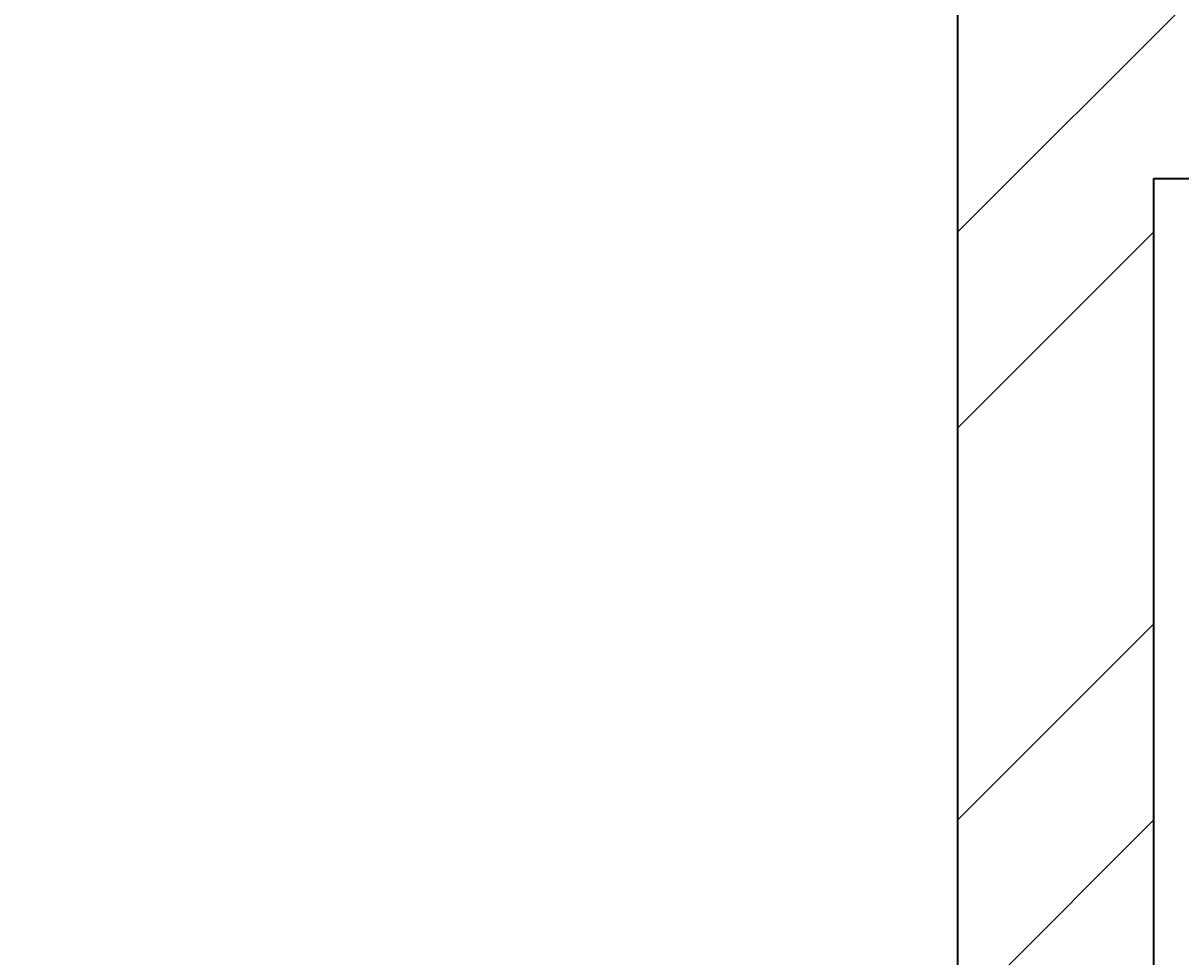
# Model space of a CAD drawing. Units: inches. Extents: x 1885 to 2748, y 783 to 2421.
# Tile 67 of 117: x 1995 to 2022, y 2000 to 2022. Entities that reach past the tile are written whole.
import ezdxf

# ---------------------------------------------------------------- set-up
doc = ezdxf.new("R2010")
doc.units = ezdxf.units.IN
doc.layers.add('A-ANNO-DIMS', color=2, linetype='Continuous', lineweight=18)
doc.layers.add('A-WALL', color=7, linetype='Continuous', lineweight=35)
doc.layers.add('A-WALL-PATT', color=85, linetype='Continuous', lineweight=13, true_color=0x58ba48)
doc.styles.get("Standard").update_dxf_attribs({"font": 'arial.ttf'})
doc.dimstyles.get("Standard").update_dxf_attribs({"dimtxt": 0.18, "dimasz": 0.18, "dimexe": 0.18, "dimexo": 0.0625, "dimgap": 0.09, "dimtad": 0, "dimtih": 1, "dimtoh": 1, "dimdec": 4, "dimzin": 0, "dimdsep": 46, "dimtxsty": 'Standard', "dimcen": 0.09, "dimadec": 0, "dimazin": 0, "dimtfac": 1, "dimtdec": 4, "dimtofl": 0, "dimtmove": 0, "dimatfit": 3, "dimfxl": 1, "dimtolj": 1, "dimtzin": 0, "dimarcsym": 0})

# ---------------------------------------------------------------- blocks, each defined once
blk = doc.blocks.new('*D48')
at = {"layer": 'A-ANNO-DIMS', "color": 0, "lineweight": -2, "transparency": 16777216}
for p, q in [((1980.711, 2348.006), (1902.844, 2348.006)), ((1903.024, 2347.826), (1903.024, 2114.937)), ((1903.024, 1881.686), (1903.024, 2114.574)), ((2016.711, 1881.506), (1902.844, 1881.506))]:
    blk.add_line(p, q, dxfattribs=at)
at = {"layer": 'A-ANNO-DIMS', "color": 0, "transparency": 16777216}
for points in [[(1902.994, 2347.826), (1903.054, 2347.826), (1903.024, 2348.006)], [(1902.994, 1881.686), (1903.054, 1881.686), (1903.024, 1881.506)]]:
    blk.add_solid(points, dxfattribs=at)
at = {"layer": 'Defpoints', "color": 0, "transparency": 16777216}
for p in [(1903.024, 2348.006), (1980.774, 2348.006), (2016.774, 1881.506)]:
    blk.add_point(p, dxfattribs=at)
at = {"layer": 'A-ANNO-DIMS', "color": 0, "transparency": 16777216, "insert": (1903.024, 2114.756), "char_height": 0.18, "attachment_point": 5}
blk.add_mtext('\\A1;466.5', dxfattribs=at)

msp = doc.modelspace()

# ---------------------------------------------------------------- hatches: boundary and pattern name
at = {"layer": 'A-WALL-PATT'}
h = msp.add_hatch(dxfattribs=at)
h.set_pattern_fill('ANSI32', color=256)
h.paths.add_polyline_path([(2007.772, 2318.006), (1980.774, 2318.006), (1980.774, 2281.215), (1985.274, 2281.215), (1985.274, 2313.506), (2007.772, 2313.506), (2007.772, 2315.756)])
h.paths.add_polyline_path([(2094.324, 2318.006), (2067.772, 2318.006), (2067.772, 2313.506), (2094.324, 2313.506), (2094.324, 2315.756)])
h.paths.add_polyline_path([(2131.367, 2315.756), (2131.367, 2318.006), (2131.189, 2318.006), (2112.609, 2318.006), (2112.609, 2313.506), (2117.274, 2313.506), (2117.274, 2255.201), (2121.774, 2255.201), (2121.774, 2313.506), (2131.367, 2313.506)])
h.paths.add_polyline_path([(2190.512, 2318.006), (2155.367, 2318.006), (2155.367, 2313.506), (2169.774, 2313.506), (2169.774, 2229.506), (2121.774, 2229.506), (2121.774, 2233.451), (2119.524, 2233.451), (2117.274, 2233.451), (2117.274, 2201.101), (2121.774, 2201.101), (2121.774, 2225.006), (2169.774, 2225.006), (2169.774, 2165.006), (2306.274, 2165.006), (2306.274, 2066.006), (2310.774, 2066.006), (2344.274, 2066.006), (2486.274, 2066.006), (2486.274, 1886.006), (2483.02, 1886.006), (2483.02, 1881.506), (2486.274, 1881.506), (2486.274, 1880.678), (2490.774, 1880.678), (2490.774, 2070.506), (2344.274, 2070.506), (2310.774, 2070.506), (2310.774, 2165.006), (2310.774, 2173.636), (2308.524, 2173.636), (2306.274, 2173.636), (2306.274, 2169.506), (2174.274, 2169.506), (2174.274, 2313.506), (2190.512, 2313.506), (2190.512, 2315.756)])
h.paths.add_polyline_path([(1985.274, 2221.215), (1980.774, 2221.215), (1980.774, 2165.006), (1992.774, 2165.006), (1992.774, 2141.927), (1997.274, 2141.927), (1997.274, 2165.006), (2117.274, 2165.006), (2117.274, 2163.126), (2121.774, 2163.126), (2121.774, 2172.734), (2119.524, 2172.734), (2117.274, 2172.734), (2117.274, 2169.506), (1985.274, 2169.506)])
h.paths.add_polyline_path([(1997.274, 2105.927), (1992.774, 2105.927), (1992.774, 2070.506), (2016.774, 2070.506), (2016.774, 2059.123), (2019.024, 2059.123), (2021.274, 2059.123), (2021.274, 2070.506), (2117.274, 2070.506), (2117.274, 2022.506), (2114.423, 2022.506), (2114.423, 2018.006), (2123.627, 2018.006), (2123.627, 2020.256), (2123.627, 2022.506), (2121.774, 2022.506), (2121.774, 2142.587), (2119.524, 2142.587), (2117.274, 2142.587), (2117.274, 2075.006), (1997.274, 2075.006)])
h.paths.add_polyline_path([(2092.029, 2020.256), (2092.029, 2022.506), (2021.274, 2022.506), (2021.274, 2035.123), (2016.774, 2035.123), (2016.774, 2018.006), (2016.774, 1978.784), (2021.274, 1978.784), (2021.274, 2018.006), (2092.029, 2018.006)])
h.paths.add_polyline_path([(2260.938, 2022.506), (2153.105, 2022.506), (2153.105, 2020.256), (2153.105, 2018.006), (2155.274, 2018.006), (2155.274, 1886.006), (2107.629, 1886.006), (2107.629, 1881.506), (2182.911, 1881.506), (2182.911, 1883.756), (2182.911, 1886.006), (2159.774, 1886.006), (2159.774, 2018.006), (2260.938, 2018.006), (2260.938, 2020.256)])
h.paths.add_polyline_path([(2047.629, 1883.756), (2047.629, 1886.006), (2021.274, 1886.006), (2021.274, 1918.784), (2019.024, 1918.784), (2016.774, 1918.784), (2016.774, 1881.506), (2047.629, 1881.506)])
h.paths.add_polyline_path([(2306.361, 1883.756), (2306.361, 1886.006), (2296.274, 1886.006), (2296.274, 1982.006), (2316.535, 1982.006), (2316.535, 1984.256), (2316.535, 1986.506), (2296.274, 1986.506), (2296.274, 2022.506), (2289.276, 2022.506), (2289.276, 2018.006), (2291.774, 2018.006), (2291.774, 1886.006), (2242.911, 1886.006), (2242.911, 1881.506), (2306.361, 1881.506)], flags=17)
h.paths.add_polyline_path([(1985.274, 1843.006), (2021.6, 1843.006), (2021.534, 1845.441), (2021.477, 1847.506), (1980.774, 1847.506), (1980.774, 1809.446), (1985.274, 1809.446)])
h.paths.add_polyline_path([(2131.482, 1845.256), (2131.482, 1847.506), (2081.534, 1847.506), (2081.534, 1843.006), (2117.274, 1843.006), (2117.274, 1784.147), (2119.524, 1784.147), (2121.774, 1784.147), (2121.774, 1843.006), (2131.482, 1843.006)])
h.paths.add_polyline_path([(2203.886, 1847.506), (2155.482, 1847.506), (2155.482, 1843.006), (2169.774, 1843.006), (2169.774, 1759.006), (2121.774, 1759.006), (2121.774, 1761.457), (2117.274, 1761.457), (2117.274, 1730.429), (2121.774, 1730.429), (2121.774, 1754.506), (2177.421, 1754.506), (2177.421, 1756.756), (2177.421, 1759.006), (2174.274, 1759.006), (2174.274, 1843.006), (2203.886, 1843.006)])
h.paths.add_polyline_path([(2335.554, 1845.256), (2335.554, 1847.506), (2239.886, 1847.506), (2239.886, 1843.006), (2306.274, 1843.006), (2306.274, 1759.006), (2199.486, 1759.006), (2199.486, 1754.506), (2310.774, 1754.506), (2310.774, 1843.006), (2335.554, 1843.006)])
h.paths.add_polyline_path([(2348.774, 2022.506), (2344.274, 2022.506), (2344.274, 1986.506), (2341.681, 1986.506), (2341.681, 1982.006), (2344.274, 1982.006), (2344.274, 1886.006), (2330.361, 1886.006), (2330.361, 1881.506), (2361.627, 1881.506), (2361.627, 1883.756), (2361.627, 1886.006), (2348.774, 1886.006)], flags=17)
h.paths.add_polyline_path([(2283.251, 2315.756), (2283.251, 2318.006), (2238.512, 2318.006), (2238.512, 2313.506), (2283.251, 2313.506)], flags=17)
h.paths.add_polyline_path([(2363.274, 2348.006), (2388.677, 2348.006), (2388.677, 2350.256), (2388.677, 2352.506), (2358.774, 2352.506), (2358.774, 2348.006), (2358.774, 2318.006), (2344.481, 2318.006), (2344.481, 2313.506), (2358.774, 2313.506), (2358.774, 2229.506), (2310.774, 2229.506), (2310.774, 2231.952), (2306.274, 2231.952), (2306.274, 2205.611), (2310.774, 2205.611), (2310.774, 2225.006), (2358.774, 2225.006), (2358.774, 2211.506), (2452.329, 2211.506), (2452.329, 2213.756), (2452.329, 2216.006), (2363.274, 2216.006), (2363.274, 2318.006)])
h.paths.add_polyline_path([(2310.774, 2313.506), (2320.481, 2313.506), (2320.481, 2315.756), (2320.481, 2318.006), (2302.728, 2318.006), (2302.728, 2313.506), (2306.274, 2313.506), (2306.274, 2251.076), (2310.774, 2251.076)], flags=17)
h.paths.add_polyline_path([(2490.774, 2352.506), (2486.274, 2352.506), (2448.677, 2352.506), (2448.677, 2348.006), (2486.274, 2348.006), (2486.274, 2318.006), (2486.274, 2216.006), (2481.78, 2216.006), (2481.78, 2211.506), (2486.274, 2211.506), (2486.274, 2165.006), (2493.289, 2165.006), (2493.289, 2167.256), (2493.289, 2169.506), (2490.774, 2169.506), (2490.774, 2313.506), (2494.429, 2313.506), (2494.429, 2318.006), (2490.774, 2318.006)])
h.paths.add_polyline_path([(2534.653, 2318.006), (2515.691, 2318.006), (2515.691, 2313.506), (2534.653, 2313.506), (2534.653, 2315.756)])
h.paths.add_polyline_path([(2618.274, 2318.006), (2594.653, 2318.006), (2594.653, 2313.506), (2613.774, 2313.506), (2613.774, 2281.706), (2618.274, 2281.706)])
h.paths.add_polyline_path([(2618.274, 2221.706), (2613.774, 2221.706), (2613.774, 2169.506), (2554.019, 2169.506), (2554.019, 2165.006), (2613.774, 2165.006), (2613.774, 2152.878), (2618.274, 2152.878)])
h.paths.add_polyline_path([(2618.274, 2128.878), (2616.024, 2128.878), (2613.774, 2128.878), (2613.774, 2117.006), (2529.774, 2117.006), (2529.774, 2165.006), (2532.848, 2165.006), (2532.848, 2169.506), (2522.867, 2169.506), (2522.867, 2165.006), (2525.274, 2165.006), (2525.274, 2117.006), (2525.274, 2112.506), (2525.274, 2108.576), (2529.774, 2108.576), (2529.774, 2112.506), (2613.774, 2112.506), (2613.774, 2080.19), (2618.274, 2080.19)])
h.paths.add_polyline_path([(2618.274, 2044.19), (2616.024, 2044.19), (2613.774, 2044.19), (2613.774, 2015.506), (2529.774, 2015.506), (2529.774, 2088.582), (2527.524, 2088.582), (2525.274, 2088.582), (2525.274, 2011.006), (2613.774, 2011.006), (2613.774, 1956.755), (2618.274, 1956.755)])
h.paths.add_polyline_path([(2618.274, 1881.506), (2618.274, 1896.755), (2613.774, 1896.755), (2613.774, 1881.506), (2613.774, 1847.506), (2592.715, 1847.506), (2592.715, 1843.006), (2613.774, 1843.006), (2613.774, 1765.006), (2613.774, 1760.506), (2609.621, 1760.506), (2609.621, 1756.006), (2613.774, 1756.006), (2613.774, 1660.006), (2608.544, 1660.006), (2608.544, 1655.506), (2613.774, 1655.506), (2613.774, 1508.158), (2618.274, 1508.158)])
h.paths.add_polyline_path([(2565.774, 1843.006), (2568.997, 1843.006), (2568.997, 1847.506), (2490.774, 1847.506), (2490.774, 1849.7), (2488.524, 1849.7), (2486.274, 1849.7), (2486.274, 1847.506), (2477.274, 1847.506), (2477.274, 1838.506), (2477.274, 1821.493), (2486.274, 1821.493), (2486.274, 1838.506), (2561.274, 1838.506), (2561.274, 1765.006), (2486.274, 1765.006), (2486.274, 1786.157), (2477.274, 1786.157), (2477.274, 1765.006), (2477.274, 1756.006), (2486.274, 1756.006), (2565.774, 1756.006), (2585.621, 1756.006), (2585.621, 1758.256), (2585.621, 1760.506), (2565.774, 1760.506), (2565.774, 1765.006)])
h.paths.add_polyline_path([(2486.274, 1651.006), (2561.274, 1651.006), (2561.274, 1567.006), (2486.274, 1567.006), (2486.274, 1591.321), (2477.274, 1591.321), (2477.274, 1567.006), (2477.274, 1558.006), (2477.274, 1555.439), (2481.774, 1555.439), (2481.774, 1558.006), (2568.653, 1558.006), (2568.653, 1560.256), (2568.653, 1562.506), (2565.774, 1562.506), (2565.774, 1655.506), (2584.544, 1655.506), (2584.544, 1657.756), (2584.544, 1660.006), (2565.774, 1660.006), (2486.274, 1660.006), (2477.274, 1660.006), (2477.274, 1651.006), (2477.274, 1632.989), (2486.274, 1632.989)])
h.paths.add_polyline_path([(2449.967, 1883.756), (2449.967, 1886.006), (2421.627, 1886.006), (2421.627, 1881.506), (2449.967, 1881.506)], flags=17)
h.paths.add_polyline_path([(2447.274, 1847.506), (2395.554, 1847.506), (2395.554, 1843.006), (2442.774, 1843.006), (2442.774, 1809.27), (2447.274, 1809.27)])
h.paths.add_polyline_path([(1985.274, 1749.446), (1980.774, 1749.446), (1980.774, 1694.504), (1985.274, 1694.504), (1985.274, 1694.506), (1986.897, 1694.506), (1986.897, 1697.78), (1986.897, 1699.006), (1985.274, 1699.006)])
h.paths.add_polyline_path([(2152.774, 1699.006), (2121.774, 1699.006), (2121.774, 1703.668), (2119.524, 1703.668), (2117.274, 1703.668), (2117.274, 1699.006), (2009.219, 1699.006), (2009.219, 1694.506), (2148.274, 1694.506), (2148.274, 1692.631), (2152.774, 1692.631)])
h.paths.add_polyline_path([(2016.274, 1694.506), (2011.774, 1694.506), (2011.774, 1558.006), (2040.806, 1558.006), (2040.806, 1560.256), (2040.806, 1562.506), (2016.274, 1562.506)])
h.paths.add_polyline_path([(2152.774, 1663.017), (2150.524, 1663.017), (2148.274, 1663.017), (2148.274, 1562.506), (2100.806, 1562.506), (2100.806, 1558.006), (2165.119, 1558.006), (2165.119, 1560.256), (2165.119, 1562.506), (2152.774, 1562.506), (2152.774, 1610.506), (2224.774, 1610.506), (2224.774, 1607.99), (2229.274, 1607.99), (2229.274, 1615.006), (2152.774, 1615.006)])
h.paths.add_polyline_path([(2238.613, 1560.256), (2238.613, 1562.506), (2229.274, 1562.506), (2229.274, 1588.756), (2227.024, 1588.763), (2224.774, 1588.771), (2224.774, 1562.506), (2189.119, 1562.506), (2189.119, 1558.006), (2238.613, 1558.006)])
h.paths.add_polyline_path([(2336.024, 1560.256), (2336.024, 1562.506), (2310.774, 1562.506), (2310.774, 1656.347), (2308.524, 1656.347), (2306.274, 1656.347), (2306.274, 1562.506), (2286.613, 1562.506), (2286.613, 1558.006), (2336.024, 1558.006)])
h.paths.add_polyline_path([(2447.274, 1690.968), (2445.024, 1690.968), (2442.774, 1690.968), (2442.774, 1687.006), (2306.274, 1687.006), (2306.274, 1680.75), (2310.774, 1680.75), (2310.774, 1682.506), (2442.774, 1682.506), (2442.774, 1562.506), (2396.024, 1562.506), (2396.024, 1558.006), (2447.274, 1558.006)])
h.paths.add_polyline_path([(2447.274, 1749.27), (2445.024, 1749.27), (2442.774, 1749.27), (2442.774, 1717.232), (2447.274, 1717.232)])
h.paths.add_polyline_path([(2044.674, 1521.756), (2044.674, 1524.006), (2007.274, 1524.006), (2007.274, 1503.49), (2009.524, 1503.49), (2011.774, 1503.49), (2011.774, 1519.506), (2044.674, 1519.506)])
h.paths.add_polyline_path([(2177.969, 1521.756), (2177.969, 1524.006), (2104.674, 1524.006), (2104.674, 1519.506), (2145.774, 1519.506), (2145.774, 1387.506), (2143.37, 1387.506), (2143.37, 1383.006), (2251.585, 1383.006), (2251.585, 1385.256), (2251.585, 1387.506), (2150.274, 1387.506), (2150.274, 1519.506), (2177.969, 1519.506)])
h.paths.add_polyline_path([(2298.704, 1524.006), (2237.969, 1524.006), (2237.969, 1519.506), (2282.274, 1519.506), (2282.274, 1387.506), (2279.683, 1387.506), (2279.683, 1383.006), (2286.774, 1383.006), (2286.774, 1419.006), (2312.451, 1419.006), (2312.451, 1421.256), (2312.451, 1423.506), (2286.774, 1423.506), (2286.774, 1519.506), (2298.704, 1519.506), (2298.704, 1521.722)], flags=17)
h.paths.add_polyline_path([(2361.897, 1521.756), (2361.897, 1524.006), (2322.704, 1524.006), (2322.704, 1519.506), (2334.774, 1519.506), (2334.774, 1423.506), (2331.93, 1423.506), (2331.93, 1419.006), (2334.774, 1419.006), (2334.774, 1387.506), (2334.774, 1383.228), (2339.274, 1383.228), (2339.274, 1387.506), (2339.274, 1519.506), (2361.897, 1519.506)], flags=17)
h.paths.add_polyline_path([(2447.274, 1521.756), (2447.274, 1524.006), (2421.897, 1524.006), (2421.897, 1519.506), (2447.274, 1519.506)], flags=17)
h.paths.add_polyline_path([(2481.774, 1529.6), (2479.524, 1529.6), (2477.274, 1529.6), (2477.274, 1524.006), (2474.489, 1524.006), (2474.489, 1519.506), (2477.274, 1519.506), (2477.274, 1334.506), (2296.774, 1334.506), (2296.774, 1240.506), (2160.274, 1240.506), (2160.274, 1180.506), (2112.274, 1180.506), (2112.274, 1207.692), (2110.024, 1207.692), (2107.774, 1207.692), (2107.774, 1171.609), (2112.274, 1171.609), (2112.274, 1176.006), (2160.274, 1176.006), (2160.274, 1092.006), (2144.221, 1092.006), (2144.221, 1087.506), (2189.497, 1087.506), (2189.497, 1089.756), (2189.497, 1092.006), (2164.774, 1092.006), (2164.774, 1236.006), (2296.774, 1236.006), (2296.774, 1231.912), (2301.274, 1231.912), (2301.274, 1330.006), (2481.774, 1330.006), (2481.774, 1387.506)])
h.paths.add_polyline_path([(2618.274, 1448.158), (2613.774, 1448.158), (2613.774, 1382.506), (2529.774, 1382.506), (2525.274, 1382.506), (2525.274, 1307.062), (2529.774, 1307.062), (2529.774, 1378.006), (2613.774, 1378.006), (2613.774, 1354.988), (2618.274, 1354.988)])
h.paths.add_polyline_path([(2618.274, 1318.988), (2613.774, 1318.988), (2613.774, 1281.006), (2529.774, 1281.006), (2529.774, 1283.786), (2527.524, 1283.786), (2525.274, 1283.786), (2525.274, 1228.506), (2516.794, 1228.506), (2516.794, 1224.006), (2533.484, 1224.006), (2533.484, 1226.256), (2533.484, 1228.506), (2529.774, 1228.506), (2529.774, 1276.506), (2613.774, 1276.506), (2613.774, 1266.02), (2618.274, 1266.02)])
h.paths.add_polyline_path([(2618.274, 1134.964), (2613.774, 1134.964), (2613.774, 1092.006), (2594.545, 1092.006), (2594.545, 1087.506), (2618.274, 1087.506)])
h.paths.add_polyline_path([(2534.545, 1092.006), (2509.765, 1092.006), (2509.765, 1087.506), (2534.545, 1087.506), (2534.545, 1089.756)])
h.paths.add_polyline_path([(2481.274, 1224.006), (2484.117, 1224.006), (2484.117, 1226.256), (2484.117, 1228.506), (2476.774, 1228.506), (2476.774, 1198.506), (2471.61, 1198.506), (2471.61, 1194.006), (2476.774, 1194.006), (2476.774, 1062.006), (2436.894, 1062.006), (2436.894, 1057.506), (2476.774, 1057.506), (2481.274, 1057.506), (2481.274, 1062.006), (2481.274, 1087.506), (2485.354, 1087.506), (2485.354, 1089.756), (2485.354, 1092.006), (2481.274, 1092.006), (2481.274, 1117.506)])
h.paths.add_polyline_path([(2439.898, 1198.506), (2349.274, 1198.506), (2349.274, 1194.006), (2349.274, 1180.506), (2301.274, 1180.506), (2301.274, 1201.896), (2299.024, 1201.896), (2296.774, 1201.896), (2296.774, 1172.335), (2299.024, 1172.335), (2301.274, 1172.335), (2301.274, 1176.006), (2349.274, 1176.006), (2349.274, 1092.006), (2334.452, 1092.006), (2334.452, 1087.506), (2349.274, 1087.506), (2349.274, 1057.506), (2353.774, 1057.506), (2376.894, 1057.506), (2376.894, 1059.756), (2376.894, 1062.006), (2353.774, 1062.006), (2353.774, 1087.506), (2353.774, 1180.506), (2353.774, 1194.006), (2439.898, 1194.006), (2439.898, 1196.256)])
h.paths.add_polyline_path([(2270.596, 1089.756), (2270.596, 1092.006), (2249.497, 1092.006), (2249.497, 1087.506), (2270.596, 1087.506)], flags=17)
h.paths.add_polyline_path([(2310.452, 1092.006), (2301.274, 1092.006), (2301.274, 1153.292), (2296.774, 1153.292), (2296.774, 1092.006), (2293.786, 1092.006), (2293.786, 1087.506), (2310.452, 1087.506), (2310.452, 1089.756)], flags=17)
h.paths.add_polyline_path([(2112.274, 1150.328), (2110.024, 1150.328), (2107.774, 1150.328), (2107.774, 1092.006), (2104.465, 1092.006), (2104.465, 1087.506), (2120.221, 1087.506), (2120.221, 1089.756), (2120.221, 1092.006), (2112.274, 1092.006)])
h.paths.add_polyline_path([(2082.172, 1092.006), (2058.144, 1092.006), (2058.144, 1087.506), (2082.172, 1087.506), (2082.172, 1089.756)])
h.paths.add_polyline_path([(1975.774, 1145.638), (1971.274, 1145.638), (1971.274, 1087.506), (1980.774, 1087.506), (1998.144, 1087.506), (1998.144, 1089.756), (1998.144, 1092.006), (1985.274, 1092.006), (1975.774, 1092.006)])
h.paths.add_polyline_path([(2112.274, 1244.385), (2110.024, 1244.385), (2107.774, 1244.385), (2107.774, 1240.506), (1992.274, 1240.506), (1992.274, 1271.008), (1987.774, 1271.008), (1987.774, 1240.506), (1980.774, 1240.506), (1975.774, 1240.506), (1971.274, 1240.506), (1971.274, 1205.638), (1975.774, 1205.638), (1975.774, 1236.006), (2107.774, 1236.006), (2107.774, 1233.444), (2112.274, 1233.444), (2112.274, 1236.006)])
h.paths.add_polyline_path([(2112.274, 1383.006), (2114.783, 1383.006), (2114.783, 1385.256), (2114.783, 1387.506), (2102.476, 1387.506), (2102.476, 1383.006), (2107.774, 1383.006), (2107.774, 1335.006), (2011.774, 1335.006), (2011.774, 1349.939), (2007.274, 1349.939), (2007.274, 1335.006), (1987.774, 1335.006), (1987.774, 1330.506), (1987.774, 1307.008), (1992.274, 1307.008), (1992.274, 1330.506), (2007.274, 1330.506), (2107.774, 1330.506), (2107.774, 1264.711), (2112.274, 1264.711)])
h.paths.add_polyline_path([(2077.857, 1387.506), (2011.774, 1387.506), (2011.774, 1390.036), (2009.524, 1390.036), (2007.274, 1390.036), (2007.274, 1373.939), (2011.774, 1373.939), (2011.774, 1383.006), (2077.857, 1383.006)])
h.paths.add_polyline_path([(2011.774, 1443.49), (2007.274, 1443.49), (2007.274, 1410.248), (2011.774, 1410.248)])

# ---------------------------------------------------------------- linework, layer by layer
at = {"layer": 'A-WALL'}
for p, q in [((2016.774, 2035.123), (2016.774, 2018.006)), ((2016.774, 2018.006), (2016.774, 1978.784)), ((2021.274, 2018.006), (2092.029, 2018.006)), ((2021.274, 1978.784), (2021.274, 2018.006))]:
    msp.add_line(p, q, dxfattribs=at)

# ---------------------------------------------------------------- dimensions: what is measured, and where the dimension line sits
at = {"layer": 'A-ANNO-DIMS'}
dim = msp.add_linear_dim(base=(1903.024, 2348.006), p1=(2016.774, 1881.506), p2=(1980.774, 2348.006), angle=90, dimstyle='Standard', override={"dimdec": 1, "dimlfac": 1, "dimrnd": 0, "dimzin": 0, "dimdsep": 46, "dimlunit": 2}, dxfattribs=at)
dim.commit()
dim.dimension.update_dxf_attribs({"geometry": '*D48', "text_midpoint": (1903.024, 2114.756)})

doc.saveas('drawing.dxf')
